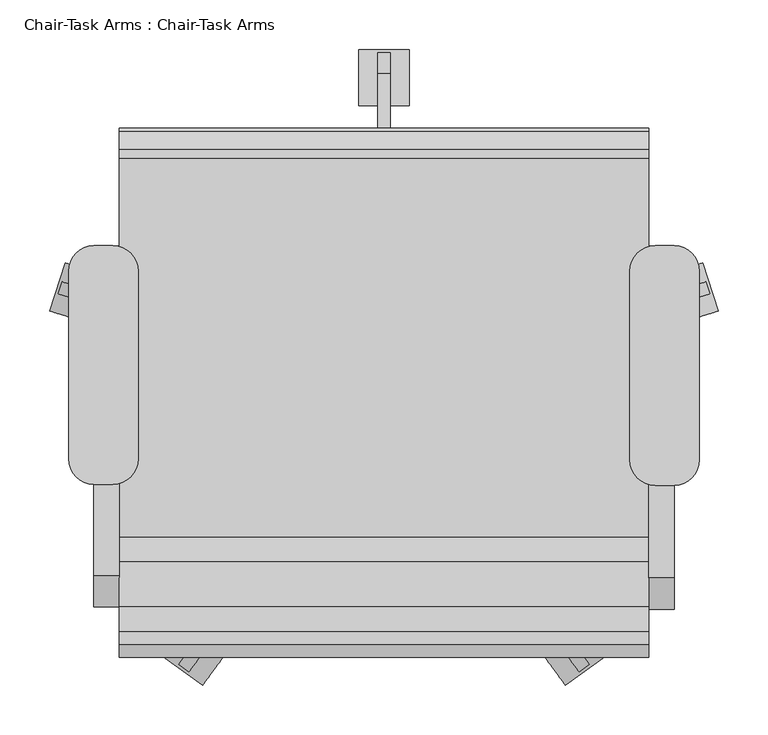
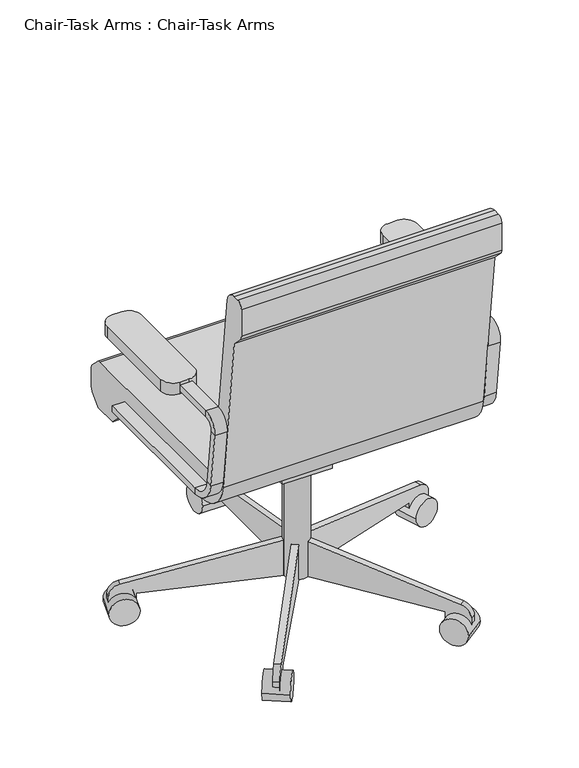
"""IFC4 building model written with IfcOpenShell, lengths in millimetres: furniture geometry, Chair-Task Arms : Chair-Task Arms."""

from ifc_helpers import new_model, si_unit, point, frame, frame_2d, origin, place, context, project, spatial, polyline, circle_curve, trimmed, segment, composite_curve, outline, extrude, source, transform, mapped, element, save
from ifc_brep_helpers import plane_surface, cylinder_surface, revolved_surface, advanced_brep


def chair_task_arms_chair_task_arms_fa5a08ef(model_context):
    return source(origin(), model_context, "Body", "SolidModel", [
        extrude(outline(composite_curve([segment(polyline([(433.0908197, -74.2028048), (414.0408197, -74.2028048)]), True, "CONTINUOUS"), segment(trimmed(circle_curve(frame_2d((414.0408197, -48.8028048)), 25.4), [point((414.0408197, -74.2028048))], [point((388.6408197, -48.8028048))], False, "CARTESIAN"), True, "CONTINUOUS"), segment(polyline([(388.6408197, -48.8028048), (388.6408197, 141.6319091)]), True, "CONTINUOUS"), segment(trimmed(circle_curve(frame_2d((414.0408197, 141.6319091)), 25.4), [point((388.6408197, 141.6319091))], [point((414.0408197, 167.0319091))], False, "CARTESIAN"), True, "CONTINUOUS"), segment(polyline([(414.0408197, 167.0319091), (433.0908197, 167.0319091)]), True, "CONTINUOUS"), segment(trimmed(circle_curve(frame_2d((433.0908197, 141.6319091)), 25.4), [point((433.0908197, 167.0319091))], [point((458.4908197, 141.6319091))], False, "CARTESIAN"), True, "CONTINUOUS"), segment(polyline([(458.4908197, 141.6319091), (458.4908197, -48.8028048)]), True, "CONTINUOUS"), segment(trimmed(circle_curve(frame_2d((433.0908197, -48.8028048)), 25.4), [point((458.4908197, -48.8028048))], [point((433.0908197, -74.2028048))], False, "CARTESIAN"), True, "CONTINUOUS")], self_intersect=False)), frame((0.0, 0.0, 596.9), z_axis=(0.0, 0.0, 1.0), x_axis=(1.0, 0.0, 0.0)), (0.0, 0.0, 1.0), 25.4),
        extrude(outline(composite_curve([segment(polyline([(-132.0591803, -73.1575984), (-151.1091803, -73.1575984)]), True, "CONTINUOUS"), segment(trimmed(circle_curve(frame_2d((-151.1091803, -47.7575984)), 25.4), [point((-151.1091803, -73.1575984))], [point((-176.5091803, -47.7575984))], False, "CARTESIAN"), True, "CONTINUOUS"), segment(polyline([(-176.5091803, -47.7575984), (-176.5091803, 141.6319091)]), True, "CONTINUOUS"), segment(trimmed(circle_curve(frame_2d((-151.1091803, 141.6319091)), 25.4), [point((-176.5091803, 141.6319091))], [point((-151.1091803, 167.0319091))], False, "CARTESIAN"), True, "CONTINUOUS"), segment(polyline([(-151.1091803, 167.0319091), (-132.0591803, 167.0319091)]), True, "CONTINUOUS"), segment(trimmed(circle_curve(frame_2d((-132.0591803, 141.6319091)), 25.4), [point((-132.0591803, 167.0319091))], [point((-106.6591803, 141.6319091))], False, "CARTESIAN"), True, "CONTINUOUS"), segment(polyline([(-106.6591803, 141.6319091), (-106.6591803, -47.7575984)]), True, "CONTINUOUS"), segment(trimmed(circle_curve(frame_2d((-132.0591803, -47.7575984)), 25.4), [point((-106.6591803, -47.7575984))], [point((-132.0591803, -73.1575984))], False, "CARTESIAN"), True, "CONTINUOUS")], self_intersect=False)), frame((0.0, 0.0, 596.9), z_axis=(0.0, 0.0, 1.0), x_axis=(1.0, 0.0, 0.0)), (0.0, 0.0, 1.0), 25.4),
        advanced_brep(
        [(-151.1091803, 167.0319091, 412.75), (-151.1091803, 167.0319091, 425.45), (-125.7091803, 167.0319091, 425.45), (-125.7091803, 167.0319091, 412.75), (-151.1091803, -126.2388651, 412.75), (-151.1091803, -126.2388651, 425.45), (-125.7091803, -126.2388651, 425.45), (-125.7091803, -126.2388651, 412.75), (-151.1091803, -170.3844094, 464.7064065), (-151.1091803, -182.9974221, 463.2225227), (-125.7091803, -170.3844094, 464.7064065), (-125.7091803, -182.9974221, 463.2225227), (-151.1091803, -196.7936301, 580.4902904), (-151.1091803, -184.1806174, 581.9741742), (-125.7091803, -184.1806174, 581.9741742), (-125.7091803, -196.7936301, 580.4902904), (-151.1091803, -165.2610984, 603.25), (-151.1091803, -165.2610984, 615.95), (-125.7091803, -165.2610984, 603.25), (-125.7091803, -165.2610984, 615.95), (-151.1091803, 18.9459016, 615.95), (-125.7091803, 18.9459016, 615.95), (-125.7091803, 18.9459016, 603.25), (-151.1091803, 18.9459016, 603.25)],
        [
            (0, 1),
            (1, 2),
            (2, 3),
            (3, 0),
            (0, 4),
            (4, 5),
            (5, 1),
            (5, 6),
            (6, 2),
            (6, 7),
            (7, 3),
            (7, 4),
            (8, 5, circle_curve(frame((-151.1091803, -126.2388651, 469.9), z_axis=(1.0, 0.0, 0.0), x_axis=(0.0, 0.0, -1.0)), 44.45)),
            (4, 9, circle_curve(frame((-151.1091803, -126.2388651, 469.9), z_axis=(-1.0, 0.0, 0.0), x_axis=(0.0, 0.0, -1.0)), 57.15)),
            (9, 8),
            (10, 6, circle_curve(frame((-125.7091803, -126.2388651, 469.9), z_axis=(1.0, 0.0, 0.0), x_axis=(0.0, 0.0, -1.0)), 44.45)),
            (8, 10),
            (11, 7, circle_curve(frame((-125.7091803, -126.2388651, 469.9), z_axis=(1.0, 0.0, 0.0), x_axis=(0.0, 0.0, -1.0)), 57.15)),
            (10, 11),
            (11, 9),
            (9, 12),
            (12, 13),
            (13, 8),
            (13, 14),
            (14, 10),
            (14, 15),
            (15, 11),
            (15, 12),
            (16, 13, circle_curve(frame((-151.1091803, -165.2610984, 584.2), z_axis=(1.0, 0.0, 0.0), x_axis=(0.0, -0.9931506043228768, -0.11684124756739202)), 19.05)),
            (12, 17, circle_curve(frame((-151.1091803, -165.2610984, 584.2), z_axis=(-1.0, 0.0, 0.0), x_axis=(0.0, -0.9931506043228768, -0.11684124756739202)), 31.75)),
            (17, 16),
            (18, 14, circle_curve(frame((-125.7091803, -165.2610984, 584.2), z_axis=(1.0, 0.0, 0.0), x_axis=(0.0, -0.9931506043228768, -0.11684124756739202)), 19.05)),
            (16, 18),
            (19, 15, circle_curve(frame((-125.7091803, -165.2610984, 584.2), z_axis=(1.0, 0.0, 0.0), x_axis=(0.0, -0.9931506043228768, -0.11684124756739202)), 31.75)),
            (18, 19),
            (19, 17),
            (20, 21),
            (21, 22),
            (22, 23),
            (23, 20),
            (17, 20),
            (23, 16),
            (22, 18),
            (21, 19),
        ],
        [
            plane_surface(frame((-152.608212, 167.0319091, 419.1), z_axis=(0.0, 1.0, 0.0), x_axis=(0.0, 0.0, -1.0))),
            plane_surface(frame((-151.1091803, 167.0319091, 412.75), z_axis=(-1.0, 0.0, 0.0), x_axis=(0.0, -1.0, 0.0))),
            plane_surface(frame((-151.1091803, 167.0319091, 425.45), z_axis=(0.0, 0.0, 1.0), x_axis=(0.0, -1.0, 0.0))),
            plane_surface(frame((-125.7091803, 167.0319091, 425.45), z_axis=(1.0, 0.0, 0.0), x_axis=(0.0, -1.0, 0.0))),
            plane_surface(frame((-125.7091803, 167.0319091, 412.75), z_axis=(0.0, 0.0, -1.0), x_axis=(0.0, -1.0, 0.0))),
            plane_surface(frame((-151.1091803, -126.2388651, 469.9), z_axis=(-1.0, 0.0, 0.0), x_axis=(0.0, 0.0, -1.0))),
            revolved_surface(polyline([(-151.1091803, -126.2388651, 425.45), (-125.7091803, -126.2388651, 425.45)]), (-138.4091803, -126.2388651, 469.9), (-1.0, 0.0, 0.0)),
            plane_surface(frame((-125.7091803, -126.2388651, 469.9), z_axis=(1.0, 0.0, 0.0), x_axis=(0.0, 0.0, -1.0))),
            cylinder_surface(frame((-138.4091803, -126.2388651, 469.9), z_axis=(-1.0, 0.0, 0.0), x_axis=(0.0, 0.0, -1.0)), 57.15),
            plane_surface(frame((-151.1091803, -182.9974221, 463.2225227), z_axis=(-1.0, 0.0, 0.0), x_axis=(0.0, -0.1168412475673856, 0.9931506043228776))),
            plane_surface(frame((-151.1091803, -170.3844094, 464.7064065), z_axis=(0.0, 0.9931506043228776, 0.1168412475673856), x_axis=(0.0, -0.1168412475673856, 0.9931506043228776))),
            plane_surface(frame((-125.7091803, -170.3844094, 464.7064065), z_axis=(1.0, 0.0, 0.0), x_axis=(0.0, -0.1168412475673856, 0.9931506043228776))),
            plane_surface(frame((-125.7091803, -182.9974221, 463.2225227), z_axis=(0.0, -0.9931506043228776, -0.1168412475673856), x_axis=(0.0, -0.1168412475673856, 0.9931506043228776))),
            plane_surface(frame((-151.1091803, -165.2610984, 584.2), z_axis=(-1.0, 0.0, 0.0), x_axis=(0.0, -0.9931506043228768, -0.11684124756739202))),
            revolved_surface(polyline([(-151.1091803, -184.1806174123508, 581.9741742338413), (-125.7091803, -184.1806174123508, 581.9741742338413)]), (-138.4091803, -165.2610984, 584.2), (-1.0, 0.0, 0.0)),
            plane_surface(frame((-125.7091803, -165.2610984, 584.2), z_axis=(1.0, 0.0, 0.0), x_axis=(0.0, -0.9931506043228768, -0.11684124756739202))),
            cylinder_surface(frame((-138.4091803, -165.2610984, 584.2), z_axis=(-1.0, 0.0, 0.0), x_axis=(0.0, -0.9931506043228768, -0.11684124756739202)), 31.75),
            plane_surface(frame((-152.608212, 18.9459016, 609.6), z_axis=(0.0, 1.0, 0.0), x_axis=(0.0, 0.0, 1.0))),
            plane_surface(frame((-151.1091803, -165.2610984, 615.95), z_axis=(-1.0, 0.0, 0.0), x_axis=(0.0, 1.0, 0.0))),
            plane_surface(frame((-151.1091803, -165.2610984, 603.25), z_axis=(0.0, 0.0, -1.0), x_axis=(0.0, 1.0, 0.0))),
            plane_surface(frame((-125.7091803, -165.2610984, 603.25), z_axis=(1.0, 0.0, 0.0), x_axis=(0.0, 1.0, 0.0))),
            plane_surface(frame((-125.7091803, -165.2610984, 615.95), z_axis=(0.0, 0.0, 1.0), x_axis=(0.0, 1.0, 0.0))),
        ],
        [
            (0, [[1, 2, 3, 4]]),
            (1, [[-1, 5, 6, 7]]),
            (2, [[-2, -7, 8, 9]]),
            (3, [[-3, -9, 10, 11]]),
            (4, [[-4, -11, 12, -5]]),
            (5, [[13, -6, 14, 15]]),
            (6, [[16, -8, -13, 17]]),
            (7, [[18, -10, -16, 19]]),
            (8, [[-14, -12, -18, 20]]),
            (9, [[-15, 21, 22, 23]]),
            (10, [[-17, -23, 24, 25]]),
            (11, [[-19, -25, 26, 27]]),
            (12, [[-20, -27, 28, -21]]),
            (13, [[29, -22, 30, 31]]),
            (14, [[32, -24, -29, 33]]),
            (15, [[34, -26, -32, 35]]),
            (16, [[-30, -28, -34, 36]]),
            (17, [[37, 38, 39, 40]]),
            (18, [[-31, 41, -40, 42]]),
            (19, [[-33, -42, -39, 43]]),
            (20, [[-35, -43, -38, 44]]),
            (21, [[-36, -44, -37, -41]]),
        ],
    ),
        advanced_brep(
        [(433.0908197, 167.0319091, 425.45), (433.0908197, 167.0319091, 412.75), (407.6908197, 167.0319091, 412.75), (407.6908197, 167.0319091, 425.45), (433.0908197, -128.329278, 425.45), (433.0908197, -128.329278, 412.75), (407.6908197, -128.329278, 412.75), (407.6908197, -128.329278, 425.45), (433.0908197, -185.0878351, 463.2225227), (433.0908197, -172.4748224, 464.7064065), (407.6908197, -185.0878351, 463.2225227), (407.6908197, -172.4748224, 464.7064065), (433.0908197, -186.2710303, 581.9741742), (433.0908197, -198.884043, 580.4902904), (407.6908197, -198.884043, 580.4902904), (407.6908197, -186.2710303, 581.9741742), (433.0908197, -167.3515113, 615.95), (433.0908197, -167.3515113, 603.25), (407.6908197, -167.3515113, 615.95), (407.6908197, -167.3515113, 603.25), (433.0908197, 18.9459016, 603.25), (407.6908197, 18.9459016, 603.25), (407.6908197, 18.9459016, 615.95), (433.0908197, 18.9459016, 615.95)],
        [
            (0, 1),
            (1, 2),
            (2, 3),
            (3, 0),
            (0, 4),
            (4, 5),
            (5, 1),
            (5, 6),
            (6, 2),
            (6, 7),
            (7, 3),
            (7, 4),
            (8, 5, circle_curve(frame((433.0908197, -128.329278, 469.9), z_axis=(1.0, 0.0, 0.0), x_axis=(0.0, 0.0, -1.0)), 57.15)),
            (4, 9, circle_curve(frame((433.0908197, -128.329278, 469.9), z_axis=(-1.0, 0.0, 0.0), x_axis=(0.0, 0.0, -1.0)), 44.45)),
            (9, 8),
            (10, 6, circle_curve(frame((407.6908197, -128.329278, 469.9), z_axis=(1.0, 0.0, 0.0), x_axis=(0.0, 0.0, -1.0)), 57.15)),
            (8, 10),
            (11, 7, circle_curve(frame((407.6908197, -128.329278, 469.9), z_axis=(1.0, 0.0, 0.0), x_axis=(0.0, 0.0, -1.0)), 44.45)),
            (10, 11),
            (11, 9),
            (9, 12),
            (12, 13),
            (13, 8),
            (13, 14),
            (14, 10),
            (14, 15),
            (15, 11),
            (15, 12),
            (16, 13, circle_curve(frame((433.0908197, -167.3515113, 584.2), z_axis=(1.0, 0.0, 0.0), x_axis=(0.0, -0.9931506043228767, -0.1168412475673929)), 31.75)),
            (12, 17, circle_curve(frame((433.0908197, -167.3515113, 584.2), z_axis=(-1.0, 0.0, 0.0), x_axis=(0.0, -0.9931506043228767, -0.1168412475673929)), 19.05)),
            (17, 16),
            (18, 14, circle_curve(frame((407.6908197, -167.3515113, 584.2), z_axis=(1.0, 0.0, 0.0), x_axis=(0.0, -0.9931506043228767, -0.1168412475673929)), 31.75)),
            (16, 18),
            (19, 15, circle_curve(frame((407.6908197, -167.3515113, 584.2), z_axis=(1.0, 0.0, 0.0), x_axis=(0.0, -0.9931506043228767, -0.1168412475673929)), 19.05)),
            (18, 19),
            (19, 17),
            (20, 21),
            (21, 22),
            (22, 23),
            (23, 20),
            (17, 20),
            (23, 16),
            (22, 18),
            (21, 19),
        ],
        [
            plane_surface(frame((406.191788, 167.0319091, 419.1), z_axis=(0.0, 1.0, 0.0), x_axis=(0.0, 0.0, -1.0))),
            plane_surface(frame((433.0908197, 167.0319091, 425.45), z_axis=(1.0, 0.0, 0.0), x_axis=(0.0, -1.0, 0.0))),
            plane_surface(frame((433.0908197, 167.0319091, 412.75), z_axis=(0.0, 0.0, -1.0), x_axis=(0.0, -1.0, 0.0))),
            plane_surface(frame((407.6908197, 167.0319091, 412.75), z_axis=(-1.0, 0.0, 0.0), x_axis=(0.0, -1.0, 0.0))),
            plane_surface(frame((407.6908197, 167.0319091, 425.45), z_axis=(0.0, 0.0, 1.0), x_axis=(0.0, -1.0, 0.0))),
            plane_surface(frame((433.0908197, -128.329278, 469.9), z_axis=(1.0, 0.0, 0.0), x_axis=(0.0, 0.0, -1.0))),
            cylinder_surface(frame((420.3908197, -128.329278, 469.9), z_axis=(-1.0, 0.0, 0.0), x_axis=(0.0, 0.0, -1.0)), 57.15),
            plane_surface(frame((407.6908197, -128.329278, 469.9), z_axis=(-1.0, 0.0, 0.0), x_axis=(0.0, 0.0, -1.0))),
            revolved_surface(polyline([(407.6908197, -128.329278, 425.45), (433.0908197, -128.329278, 425.45)]), (420.3908197, -128.329278, 469.9), (-1.0, 0.0, 0.0)),
            plane_surface(frame((433.0908197, -172.4748224, 464.7064065), z_axis=(1.0, 0.0, 0.0), x_axis=(0.0, -0.11684124756738626, 0.9931506043228775))),
            plane_surface(frame((433.0908197, -185.0878351, 463.2225227), z_axis=(0.0, -0.9931506043228775, -0.11684124756738655), x_axis=(0.0, -0.11684124756738655, 0.9931506043228775))),
            plane_surface(frame((407.6908197, -185.0878351, 463.2225227), z_axis=(-1.0, 0.0, 0.0), x_axis=(0.0, -0.11684124756738626, 0.9931506043228775))),
            plane_surface(frame((407.6908197, -172.4748224, 464.7064065), z_axis=(0.0, 0.9931506043228775, 0.11684124756738626), x_axis=(0.0, -0.11684124756738626, 0.9931506043228775))),
            plane_surface(frame((433.0908197, -167.3515113, 584.2), z_axis=(1.0, 0.0, 0.0), x_axis=(0.0, -0.9931506043228767, -0.1168412475673929))),
            cylinder_surface(frame((420.3908197, -167.3515113, 584.2), z_axis=(-1.0, 0.0, 0.0), x_axis=(0.0, -0.9931506043228767, -0.1168412475673929)), 31.75),
            plane_surface(frame((407.6908197, -167.3515113, 584.2), z_axis=(-1.0, 0.0, 0.0), x_axis=(0.0, -0.9931506043228767, -0.1168412475673929))),
            revolved_surface(polyline([(407.6908197, -186.2710303123508, 581.9741742338412), (433.0908197, -186.2710303123508, 581.9741742338412)]), (420.3908197, -167.3515113, 584.2), (-1.0, 0.0, 0.0)),
            plane_surface(frame((406.191788, 18.9459016, 609.6), z_axis=(0.0, 1.0, 0.0), x_axis=(0.0, 0.0, 1.0))),
            plane_surface(frame((433.0908197, -167.3515113, 603.25), z_axis=(1.0, 0.0, 0.0), x_axis=(0.0, 1.0, 0.0))),
            plane_surface(frame((433.0908197, -167.3515113, 615.95), z_axis=(0.0, 0.0, 1.0), x_axis=(0.0, 1.0, 0.0))),
            plane_surface(frame((407.6908197, -167.3515113, 615.95), z_axis=(-1.0, 0.0, 0.0), x_axis=(0.0, 1.0, 0.0))),
            plane_surface(frame((407.6908197, -167.3515113, 603.25), z_axis=(0.0, 0.0, -1.0), x_axis=(0.0, 1.0, 0.0))),
        ],
        [
            (0, [[1, 2, 3, 4]]),
            (1, [[-1, 5, 6, 7]]),
            (2, [[-2, -7, 8, 9]]),
            (3, [[-3, -9, 10, 11]]),
            (4, [[-4, -11, 12, -5]]),
            (5, [[13, -6, 14, 15]]),
            (6, [[16, -8, -13, 17]]),
            (7, [[18, -10, -16, 19]]),
            (8, [[-14, -12, -18, 20]]),
            (9, [[-15, 21, 22, 23]]),
            (10, [[-17, -23, 24, 25]]),
            (11, [[-19, -25, 26, 27]]),
            (12, [[-20, -27, 28, -21]]),
            (13, [[29, -22, 30, 31]]),
            (14, [[32, -24, -29, 33]]),
            (15, [[34, -26, -32, 35]]),
            (16, [[-30, -28, -34, 36]]),
            (17, [[37, 38, 39, 40]]),
            (18, [[-31, 41, -40, 42]]),
            (19, [[-33, -42, -39, 43]]),
            (20, [[-35, -43, -38, 44]]),
            (21, [[-36, -44, -37, -41]]),
        ],
    ),
        extrude(outline(composite_curve([segment(trimmed(circle_curve(frame_2d((140.9908197, 18.9459016)), 25.4), [point((115.5908197, 18.9459016))], [point((166.3908197, 18.9459016))], False, "CARTESIAN"), True, "CONTINUOUS"), segment(trimmed(circle_curve(frame_2d((140.9908197, 18.9459016)), 25.4), [point((166.3908197, 18.9459016))], [point((115.5908197, 18.9459016))], False, "CARTESIAN"), True, "CONTINUOUS")], self_intersect=False)), frame((0.0, 0.0, 53.5835944), z_axis=(0.0, 0.0, 1.0), x_axis=(1.0, 0.0, 0.0)), (0.0, 0.0, 1.0), 330.5914056),
        extrude(outline(composite_curve([segment(trimmed(circle_curve(frame_2d((0.0, -28.2002727)), 28.2002727), [point((0.0, -56.4005455))], [point((0.0, 0.0))], False, "CARTESIAN"), True, "CONTINUOUS"), segment(trimmed(circle_curve(frame_2d((0.0, -28.2002727)), 28.2002727), [point((0.0, 0.0))], [point((0.0, -56.4005455))], False, "CARTESIAN"), True, "CONTINUOUS")], self_intersect=False)), frame((477.6203484, 101.6163254, 28.1835944), z_axis=(-0.3090169943749423, 0.9510565162951553, 0.0), x_axis=(0.0, 0.0, 1.0)), (0.0, 0.0, 1.0), 50.8),
        extrude(outline(composite_curve([segment(polyline([(-25.4, 0.0), (0.0, 0.0), (0.0, -50.8), (-24.303053, -50.8)]), True, "CONTINUOUS"), segment(trimmed(circle_curve(frame_2d((-24.303053, -25.4)), 25.4), [point((-24.303053, -50.8))], [point((-49.3171699, -29.8106637))], False, "CARTESIAN"), True, "CONTINUOUS"), segment(polyline([(-49.3171699, -29.8106637), (-101.6, 266.7), (-101.6, 292.1), (-25.4, 292.1), (-25.4, 0.0)]), True, "CONTINUOUS")], self_intersect=False)), frame((420.756686, 103.1705568, 28.1835944), z_axis=(-0.3090169943749423, 0.9510565162951553, 0.0), x_axis=(0.0, 0.0, -1.0)), (0.0, 0.0, 1.0), 12.7),
        extrude(outline(composite_curve([segment(trimmed(circle_curve(frame_2d((0.0, -28.2002727)), 28.2002727), [point((0.0, -56.4005455))], [point((0.0, 0.0))], False, "CARTESIAN"), True, "CONTINUOUS"), segment(trimmed(circle_curve(frame_2d((0.0, -28.2002727)), 28.2002727), [point((0.0, 0.0))], [point((0.0, -56.4005455))], False, "CARTESIAN"), True, "CONTINUOUS")], self_intersect=False)), frame((323.63931, -275.6612394, 28.1835944), z_axis=(0.8090169943749499, 0.5877852522924699, 0.0), x_axis=(0.0, 0.0, 1.0)), (0.0, 0.0, 1.0), 50.8),
        extrude(outline(composite_curve([segment(polyline([(-25.4, 0.0), (0.0, 0.0), (0.0, -50.8), (-24.303053, -50.8)]), True, "CONTINUOUS"), segment(trimmed(circle_curve(frame_2d((-24.303053, -25.3999999)), 25.4), [point((-24.303053, -50.8))], [point((-49.3171699, -29.8106636))], False, "CARTESIAN"), True, "CONTINUOUS"), segment(polyline([(-49.3171699, -29.8106636), (-101.6, 266.7), (-101.6, 292.1), (-25.4, 292.1), (-25.4, 0.0)]), True, "CONTINUOUS")], self_intersect=False)), frame((307.545634, -221.1003988, 28.1835944), z_axis=(0.8090169943749499, 0.5877852522924699, 0.0), x_axis=(0.0, 0.0, -1.0)), (0.0, 0.0, 1.0), 12.7),
        extrude(outline(composite_curve([segment(trimmed(circle_curve(frame_2d((0.0, -28.2002727)), 28.2002727), [point((0.0, -56.4005455))], [point((0.0, 0.0))], False, "CARTESIAN"), True, "CONTINUOUS"), segment(trimmed(circle_curve(frame_2d((0.0, -28.2002727)), 28.2002727), [point((0.0, 0.0))], [point((0.0, -56.4005455))], False, "CARTESIAN"), True, "CONTINUOUS")], self_intersect=False)), frame((-41.6576707, -275.6612394, 28.1835944), z_axis=(-0.8090169943749458, 0.5877852522924754, 0.0), x_axis=(0.0, 0.0, -1.0)), (0.0, 0.0, 1.0), 50.8),
        extrude(outline(composite_curve([segment(polyline([(25.4, 0.0), (25.4, 292.1), (101.6, 292.1), (101.6, 266.7), (49.3171699, -29.8106637)]), True, "CONTINUOUS"), segment(trimmed(circle_curve(frame_2d((24.303053, -25.3999999)), 25.4), [point((49.3171699, -29.8106637))], [point((24.303053, -50.8))], False, "CARTESIAN"), True, "CONTINUOUS"), segment(polyline([(24.303053, -50.8), (0.0, -50.8), (0.0, 0.0), (25.4, 0.0)]), True, "CONTINUOUS")], self_intersect=False)), frame((-25.5639946, -221.1003988, 28.1835944), z_axis=(-0.8090169943749459, 0.5877852522924754, 0.0), x_axis=(0.0, 0.0, 1.0)), (0.0, 0.0, 1.0), 12.7),
        extrude(outline(composite_curve([segment(trimmed(circle_curve(frame_2d((0.0, -28.2002727)), 28.2002727), [point((0.0, -56.4005454))], [point((0.0, 0.0))], False, "CARTESIAN"), True, "CONTINUOUS"), segment(trimmed(circle_curve(frame_2d((0.0, -28.2002727)), 28.2002727), [point((0.0, 0.0))], [point((0.0, -56.4005454))], False, "CARTESIAN"), True, "CONTINUOUS")], self_intersect=False)), frame((-195.638709, 101.6163254, 28.1835944), z_axis=(0.3090169943749487, 0.9510565162951532, 0.0), x_axis=(0.0, 0.0, -1.0)), (0.0, 0.0, 1.0), 50.8),
        extrude(outline(composite_curve([segment(polyline([(25.4, 0.0), (25.4, 292.1000001), (101.6, 292.1000001), (101.6, 266.7), (49.3171699, -29.8106636)]), True, "CONTINUOUS"), segment(trimmed(circle_curve(frame_2d((24.303053, -25.4)), 25.4), [point((49.3171699, -29.8106636))], [point((24.303053, -50.8))], False, "CARTESIAN"), True, "CONTINUOUS"), segment(polyline([(24.303053, -50.8), (0.0, -50.8), (0.0, 0.0), (25.4, 0.0)]), True, "CONTINUOUS")], self_intersect=False)), frame((-138.7750467, 103.1705568, 28.1835944), z_axis=(0.3090169943749487, 0.9510565162951532, 0.0), x_axis=(0.0, 0.0, 1.0)), (0.0, 0.0, 1.0), 12.7),
        extrude(outline(composite_curve([segment(trimmed(circle_curve(frame_2d((336.4459016, 28.1835944)), 28.2002727), [point((308.2456289, 28.1835944))], [point((364.6461744, 28.1835944))], False, "CARTESIAN"), True, "CONTINUOUS"), segment(trimmed(circle_curve(frame_2d((336.4459016, 28.1835944)), 28.2002727), [point((364.6461744, 28.1835944))], [point((308.2456289, 28.1835944))], False, "CARTESIAN"), True, "CONTINUOUS")], self_intersect=False)), frame((115.5908197, 0.0, 0.0), z_axis=(1.0, 0.0, 0.0), x_axis=(0.0, 1.0, 0.0)), (0.0, 0.0, 1.0), 50.8),
        extrude(outline(composite_curve([segment(polyline([(311.0459016, 53.5835944), (18.9459016, 53.5835944), (18.9459016, 129.7835944), (44.3459016, 129.7835944), (340.8565654, 77.5007643)]), True, "CONTINUOUS"), segment(trimmed(circle_curve(frame_2d((336.4459016, 52.4866474)), 25.4), [point((340.8565654, 77.5007643))], [point((361.8459016, 52.4866474))], False, "CARTESIAN"), True, "CONTINUOUS"), segment(polyline([(361.8459016, 52.4866474), (361.8459016, 28.1835944), (311.0459016, 28.1835944), (311.0459016, 53.5835944)]), True, "CONTINUOUS")], self_intersect=False)), frame((134.6408197, 0.0, 0.0), z_axis=(1.0, 0.0, 0.0), x_axis=(0.0, 1.0, 0.0)), (0.0, 0.0, 1.0), 12.7),
        extrude(outline(polyline([(69.7459016, 383.7835944), (69.7459016, 371.0835944), (18.9459016, 283.0954134), (-19.1540984, 283.0954134), (-19.1540984, 383.7835944), (69.7459016, 383.7835944)])), frame((90.1908197, 0.0, 0.0), z_axis=(1.0, 0.0, 0.0), x_axis=(0.0, 1.0, 0.0)), (0.0, 0.0, 1.0), 101.6),
        extrude(outline(composite_curve([segment(polyline([(-126.2050455, 457.2), (255.0102301, 457.2)]), True, "CONTINUOUS"), segment(trimmed(circle_curve(frame_2d((255.0102301, 444.5)), 12.7), [point((255.0102301, 457.2))], [point((263.9604301, 453.510212))], False, "CARTESIAN"), True, "CONTINUOUS"), segment(polyline([(263.9604301, 453.510212), (281.8961016, 435.6939999)]), True, "CONTINUOUS"), segment(trimmed(circle_curve(frame_2d((272.9459016, 426.6837879)), 12.7), [point((281.8961016, 435.6939999))], [point((285.6459016, 426.6837879))], False, "CARTESIAN"), True, "CONTINUOUS"), segment(polyline([(285.6459016, 426.6837879), (285.6459016, 391.6405184)]), True, "CONTINUOUS"), segment(trimmed(circle_curve(frame_2d((260.2459016, 391.6405184)), 25.4), [point((285.6459016, 391.6405184))], [point((278.2663256, 373.7401184))], False, "CARTESIAN"), True, "CONTINUOUS"), segment(polyline([(278.2663256, 373.7401184), (260.2470284, 355.6), (209.4470284, 355.6), (181.0744602, 383.7835944), (-107.1089978, 383.7835944)]), True, "CONTINUOUS"), segment(trimmed(circle_curve(frame_2d((-107.1089978, 459.9835944)), 76.2), [point((-107.1089978, 383.7835944))], [point((-182.7870738, 451.0802913))], False, "CARTESIAN"), True, "CONTINUOUS"), segment(polyline([(-182.7870738, 451.0802913), (-222.3540984, 787.4), (-244.0343545, 809.0802561)]), True, "CONTINUOUS"), segment(trimmed(circle_curve(frame_2d((-235.0540984, 818.0605122)), 12.7), [point((-244.0343545, 809.0802561))], [point((-247.7540984, 818.0605122))], False, "CARTESIAN"), True, "CONTINUOUS"), segment(polyline([(-247.7540984, 818.0605122), (-247.7540984, 876.3)]), True, "CONTINUOUS"), segment(trimmed(circle_curve(frame_2d((-235.0540984, 876.3)), 12.7), [point((-247.7540984, 876.3))], [point((-235.0540984, 889.0))], False, "CARTESIAN"), True, "CONTINUOUS"), segment(polyline([(-235.0540984, 889.0), (-222.1789239, 889.0)]), True, "CONTINUOUS"), segment(trimmed(circle_curve(frame_2d((-222.1789239, 863.6)), 25.4), [point((-222.1789239, 889.0))], [point((-196.9528985, 866.5677677))], False, "CARTESIAN"), True, "CONTINUOUS"), segment(polyline([(-196.9528985, 866.5677677), (-151.4310708, 479.6322323)]), True, "CONTINUOUS"), segment(trimmed(circle_curve(frame_2d((-126.2050455, 482.6)), 25.4), [point((-151.4310708, 479.6322323))], [point((-126.2050455, 457.2))], True, "CARTESIAN"), True, "CONTINUOUS")], self_intersect=False)), frame((-125.7091803, 0.0, 0.0), z_axis=(1.0, 0.0, 0.0), x_axis=(0.0, 1.0, 0.0)), (0.0, 0.0, 1.0), 533.4),
    ])


if __name__ == "__main__":
    model = new_model("IFC4")
    model_context = context("Model", 3, world=origin())
    ifc_project = project(units=[si_unit("LENGTHUNIT", "METRE", prefix="MILLI")], contexts=[model_context])
    site = spatial("IfcSite", under=ifc_project)
    building = spatial("IfcBuilding", under=site)
    placement = place(None, origin())
    chair_task_arms_chair_task_arms_shape = chair_task_arms_chair_task_arms_fa5a08ef(model_context)
    element("IfcFurniture", 1, ObjectType="Chair-Task Arms : Chair-Task Arms", at=placement, inside=building, context=model_context, shape_type="MappedRepresentation", body=[
        mapped(chair_task_arms_chair_task_arms_shape, transform((0.0, 0.0, 0.0), x_axis=(1.0, 0.0, 0.0), y_axis=(0.0, 1.0, 0.0), z_axis=(0.0, 0.0, 1.0))),
    ])
    save(model, "model.ifc")

# Revit data of these elements
# Type "Chair-Task Arms : Chair-Task Arms"
#   Assembly Code = "E2020200"
#   Base Material = Plastic - Black
#   Caster Material = Plastic - Black
#   Seat/Back Material = Textile - Slate Blue
#   Default Elevation = 0
# Element 1 (IfcFurniture, "Chair-Task Arms : Chair-Task Arms")
#   Materials on its faces: "Plastic - Black", "Textile - Slate Blue"
# Materials
#   "Plastic - Black": colour RGB 0 0 0, transparency 0.7
#   "Textile - Slate Blue": class "Fabric", colour RGB 98 102 118, transparency 0
